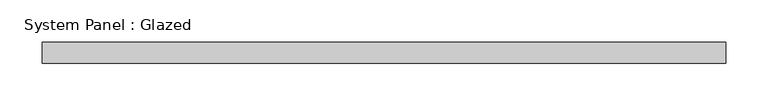
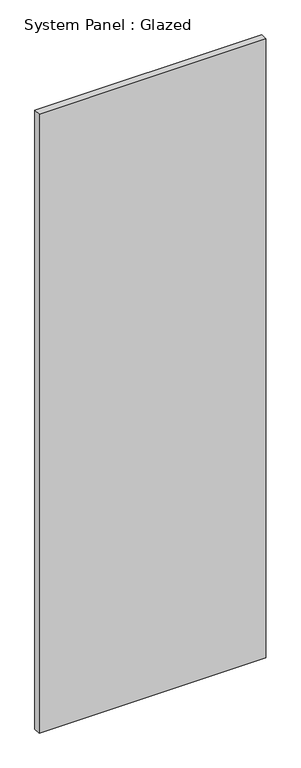
"""IFC4 building model written with IfcOpenShell, lengths in millimetres: plate geometry, System Panel : Glazed."""

from ifc_helpers import new_model, si_unit, origin, origin_with_axes, place, context, project, spatial, polyline, outline, extrude, source, transform, mapped, element, save


def system_panel_glazed_a6494cf1(model_context):
    return source(origin(), model_context, "Body", "SweptSolid", [
        extrude(outline(polyline([(406.4, 19.05), (-406.4, 19.05), (-406.4, 44.45), (406.4, 44.45), (406.4, 19.05)])), origin_with_axes(), (0.0, 0.0, 1.0), 2343.15),
    ])


if __name__ == "__main__":
    model = new_model("IFC4")
    model_context = context("Model", 3, world=origin())
    ifc_project = project(units=[si_unit("LENGTHUNIT", "METRE", prefix="MILLI")], contexts=[model_context])
    site = spatial("IfcSite", under=ifc_project)
    building = spatial("IfcBuilding", under=site)
    placement = place(None, origin())
    system_panel_glazed_shape = system_panel_glazed_a6494cf1(model_context)
    element("IfcPlate", 1, ObjectType="System Panel : Glazed", at=placement, inside=building, context=model_context, shape_type="MappedRepresentation", body=[
        mapped(system_panel_glazed_shape, transform((0.0, 0.0, 0.0), x_axis=(1.0, 0.0, 0.0), y_axis=(0.0, 1.0, 0.0), z_axis=(0.0, 0.0, 1.0))),
    ])
    save(model, "model.ifc")

# Revit data of these elements
# Type "System Panel : Glazed"
#   Construction Type Id = "GSP4R"
#   Analytic Construction = "1/8 in Pilkington single glazing"
#   Visual Light Transmittance = 0.9
#   Solar Heat Gain Coefficient = 0.86
#   Heat Transfer Coefficient (U) = 1.18115 BTU/(h·ft²·°F)
#   Define Thermal Properties by = 1
# Element 1 (IfcPlate, "System Panel : Glazed")
#   Materials on its faces: "Glass"
# Materials
#   "Glass": class "Glass", colour RGB 0 128 192, transparency 0.75, Description = "Soda Lime Glass", Cost = 0
